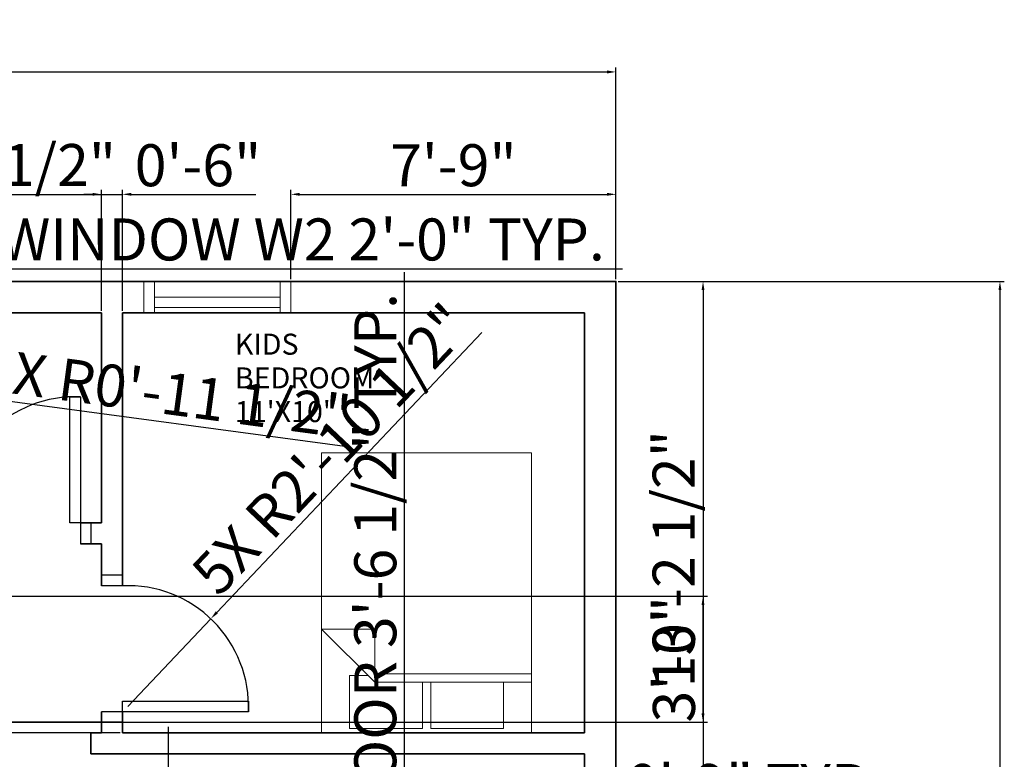
# Model space of a CAD drawing. Units: inches. Extents: x 2330 to 2931, y 514 to 1098.
# Tile 4 of 4: x 2583 to 2865, y 885 to 1096. Entities that reach past the tile are written whole.
import ezdxf

# ---------------------------------------------------------------- set-up
doc = ezdxf.new("R2010")
doc.units = ezdxf.units.IN
for name, color, linetype, lineweight in [('A-ANNO-DIMS', 2, 'Continuous', 18), ('A-AREA-IDEN', 7, 'Continuous', 18), ('A-DOOR', 3, 'Continuous', 25), ('A-FURN', 8, 'Continuous', 18), ('A-GLAZ', 4, 'Continuous', 18), ('A-WALL', 7, 'Continuous', 35)]:
    doc.layers.add(name, color=color, linetype=linetype, lineweight=lineweight)
doc.styles.get("Standard").update_dxf_attribs({"font": 'arial.ttf'})
doc.dimstyles.new('ISO-25', dxfattribs={"dimtxt": 12, "dimasz": 2.5, "dimexe": 1.25, "dimexo": 0.625, "dimtad": 1, "dimdec": 1, "dimlunit": 3, "dimtxsty": 'Standard', "dimcen": 2.5, "dimadec": 0, "dimazin": 0, "dimtfac": 1, "dimtdec": 1, "dimtmove": 0, "dimatfit": 3, "dimfxl": 1, "dimarcsym": 0})

# ---------------------------------------------------------------- blocks, each defined once
blk = doc.blocks.new('*D1')
at = {"layer": 'A-ANNO-DIMS', "color": 0, "lineweight": -2, "transparency": 16777216}
for p, q in [((2381.8, 1022.1), (2381.8, 1082.6)), ((2384.3, 1081.35), (2751.3, 1081.35)), ((2753.8, 1022.1), (2753.8, 1082.6))]:
    blk.add_line(p, q, dxfattribs=at)
at = {"layer": 'A-ANNO-DIMS', "color": 0, "transparency": 16777216}
for points in [[(2384.3, 1081.77), (2384.3, 1080.93), (2381.8, 1081.35)], [(2751.3, 1081.77), (2751.3, 1080.93), (2753.8, 1081.35)]]:
    blk.add_solid(points, dxfattribs=at)
at = {"layer": 'Defpoints', "color": 0, "transparency": 16777216}
for p in [(2753.8, 1081.35), (2381.8, 1021.47), (2753.8, 1021.47)]:
    blk.add_point(p, dxfattribs=at)
at = {"layer": 'A-ANNO-DIMS', "color": 0, "transparency": 16777216, "insert": (2567.8, 1088.11), "char_height": 12, "attachment_point": 5}
blk.add_mtext("31'", dxfattribs=at)
blk = doc.blocks.new('*D2')
at = {"layer": 'A-ANNO-DIMS', "color": 0, "lineweight": -2, "transparency": 16777216}
for p, q in [((2754.43, 1021.47), (2864.79, 1021.47)), ((2863.54, 1018.97), (2863.54, 600.97)), ((2754.43, 598.47), (2864.79, 598.47))]:
    blk.add_line(p, q, dxfattribs=at)
at = {"layer": 'A-ANNO-DIMS', "color": 0, "transparency": 16777216}
for points in [[(2863.12, 1018.97), (2863.96, 1018.97), (2863.54, 1021.47)], [(2863.12, 600.97), (2863.96, 600.97), (2863.54, 598.47)]]:
    blk.add_solid(points, dxfattribs=at)
at = {"layer": 'Defpoints', "color": 0, "transparency": 16777216}
for p in [(2753.8, 1021.47), (2753.8, 598.47), (2863.54, 598.47)]:
    blk.add_point(p, dxfattribs=at)
at = {"layer": 'A-ANNO-DIMS', "color": 0, "transparency": 16777216, "insert": (2856.78, 809.97), "char_height": 12, "attachment_point": 5, "rotation": 90}
blk.add_mtext('35\'-3"', dxfattribs=at)
blk = doc.blocks.new('Bed - Queen')
for p, q in [((0, -80.00003), (0, 0)), ((0, 0), (59.99999, 0)), ((59.99999, 0), (59.99999, -80.00003)), ((7.99999, -1.2), (28.79998, -1.2)), ((7.99999, -14.4), (7.99999, -1.2)), ((28.79998, -1.2), (28.79998, -14.4)), ((31.19999, -1.2), (51.99999, -1.2)), ((31.19999, -14.4), (31.19999, -1.2)), ((51.99999, -1.2), (51.99999, -16.4)), ((0, -14.4), (44.8, -14.4)), ((44.8, -16.8), (0, -16.8)), ((59.99999, -29.6), (44.8, -14.4)), ((44.8, -14.4), (44.8, -29.6)), ((51.99999, -16.4), (46.79936, -16.4)), ((44.8, -29.6), (59.99999, -29.6)), ((59.99999, -80.00003), (0, -80.00003))]:
    blk.add_line(p, q)
blk = doc.blocks.new('DOOR-SWING-36IN')
for p, q in [((0, 6), (0, 0)), ((3, 6), (3, 0)), ((39, 6), (39, 0)), ((42, 6), (42, 0))]:
    blk.add_line(p, q)
blk.add_lwpolyline([(39, 6), (36, 6), (36, 42), (39, 42)], close=True)
blk.add_arc((37.5, 7.5), 34.53, 87.5104, 182.4896)
blk = doc.blocks.new('WIN-36IN')
for p, q in [((0, 9), (0, 0)), ((39, 9), (3, 9)), ((3, 9), (3, 0)), ((39, 0), (39, 9)), ((42, 0), (42, 9)), ((3, 4.5), (39, 4.5)), ((3, 1.5), (39, 1.5)), ((3, 0), (39, 0))]:
    blk.add_line(p, q)
blk = doc.blocks.new('*D15')
at = {"layer": 'A-ANNO-DIMS', "color": 0, "lineweight": -2, "transparency": 16777216}
for p, q in [((2693.44, 802.89), (2693.44, 1024.11)), ((2699.18, 802.89), (2692.19, 802.89)), ((2693.44, 762.97), (2693.44, 800.39)), ((2699.18, 760.47), (2692.19, 760.47))]:
    blk.add_line(p, q, dxfattribs=at)
at = {"layer": 'A-ANNO-DIMS', "color": 0, "transparency": 16777216}
for points in [[(2693.02, 800.39), (2693.86, 800.39), (2693.44, 802.89)], [(2693.02, 762.97), (2693.86, 762.97), (2693.44, 760.47)]]:
    blk.add_solid(points, dxfattribs=at)
at = {"layer": 'Defpoints', "color": 0, "transparency": 16777216}
for p in [(2693.44, 802.89), (2699.8, 802.89), (2699.8, 760.47)]:
    blk.add_point(p, dxfattribs=at)
at = {"layer": 'A-ANNO-DIMS', "color": 0, "transparency": 16777216, "insert": (2686.6, 914.75), "char_height": 12, "attachment_point": 5, "rotation": 90}
blk.add_mtext('SWING DOOR 3\'-6 1/2" TYP.', dxfattribs=at)
blk = doc.blocks.new('*D18')
at = {"layer": 'A-ANNO-DIMS', "color": 0, "lineweight": -2, "transparency": 16777216}
for p, q in [((2744.8, 863.55), (2744.8, 870.47)), ((2753.8, 863.55), (2753.8, 870.47)), ((2747.3, 869.22), (2751.3, 869.22)), ((2753.8, 869.22), (2830.7, 869.22))]:
    blk.add_line(p, q, dxfattribs=at)
at = {"layer": 'A-ANNO-DIMS', "color": 0, "transparency": 16777216}
for points in [[(2747.3, 869.64), (2747.3, 868.8), (2744.8, 869.22)], [(2751.3, 869.64), (2751.3, 868.8), (2753.8, 869.22)]]:
    blk.add_solid(points, dxfattribs=at)
at = {"layer": 'Defpoints', "color": 0, "transparency": 16777216}
for p in [(2753.8, 869.22), (2744.8, 862.92), (2753.8, 862.92)]:
    blk.add_point(p, dxfattribs=at)
at = {"layer": 'A-ANNO-DIMS', "color": 0, "transparency": 16777216, "insert": (2793.5, 875.97), "char_height": 12, "attachment_point": 5}
blk.add_mtext('0\'-9" TYP.', dxfattribs=at)
blk = doc.blocks.new('*D19')
at = {"layer": 'A-ANNO-DIMS', "color": 0, "lineweight": -2, "transparency": 16777216}
for p, q in [((2546.27, 1022.1), (2546.27, 1026.32)), ((2548.77, 1025.07), (2567.77, 1025.07)), ((2570.27, 1022.1), (2570.27, 1026.32)), ((2570.27, 1025.07), (2755.68, 1025.07))]:
    blk.add_line(p, q, dxfattribs=at)
at = {"layer": 'A-ANNO-DIMS', "color": 0, "transparency": 16777216}
for points in [[(2548.77, 1025.49), (2548.77, 1024.66), (2546.27, 1025.07)], [(2567.77, 1025.49), (2567.77, 1024.66), (2570.27, 1025.07)]]:
    blk.add_solid(points, dxfattribs=at)
at = {"layer": 'Defpoints', "color": 0, "transparency": 16777216}
for p in [(2570.27, 1025.07), (2546.27, 1021.47), (2570.27, 1021.47)]:
    blk.add_point(p, dxfattribs=at)
at = {"layer": 'A-ANNO-DIMS', "color": 0, "transparency": 16777216, "insert": (2664.23, 1031.91), "char_height": 12, "attachment_point": 5}
blk.add_mtext('WINDOW W2 2\'-0" TYP.', dxfattribs=at)
blk = doc.blocks.new('*D39')
at = {"layer": 'A-ANNO-DIMS', "color": 0, "lineweight": -2, "transparency": 16777216}
for p, q in [((2606.8, 1013.1), (2606.8, 1047.61)), ((2612.8, 1013.1), (2612.8, 1047.61)), ((2604.3, 1046.36), (2601.8, 1046.36)), ((2606.8, 1046.36), (2612.8, 1046.36)), ((2615.3, 1046.36), (2650.95, 1046.36))]:
    blk.add_line(p, q, dxfattribs=at)
at = {"layer": 'A-ANNO-DIMS', "color": 0, "transparency": 16777216}
for points in [[(2604.3, 1046.78), (2604.3, 1045.95), (2606.8, 1046.36)], [(2615.3, 1046.78), (2615.3, 1045.95), (2612.8, 1046.36)]]:
    blk.add_solid(points, dxfattribs=at)
at = {"layer": 'Defpoints', "color": 0, "transparency": 16777216}
for p in [(2612.8, 1046.36), (2606.8, 1012.47), (2612.8, 1012.47)]:
    blk.add_point(p, dxfattribs=at)
at = {"layer": 'A-ANNO-DIMS', "color": 0, "transparency": 16777216, "insert": (2634.38, 1053.12), "char_height": 12, "attachment_point": 5}
blk.add_mtext('0\'-6"', dxfattribs=at)
blk = doc.blocks.new('*D40')
at = {"layer": 'A-ANNO-DIMS', "color": 0, "lineweight": -2, "transparency": 16777216}
for p, q in [((2528.8, 1013.1), (2528.8, 1047.61)), ((2546.27, 1013.1), (2546.27, 1047.61)), ((2531.3, 1046.36), (2543.77, 1046.36)), ((2546.27, 1046.36), (2608.76, 1046.36))]:
    blk.add_line(p, q, dxfattribs=at)
at = {"layer": 'A-ANNO-DIMS', "color": 0, "transparency": 16777216}
for points in [[(2531.3, 1046.78), (2531.3, 1045.95), (2528.8, 1046.36)], [(2543.77, 1046.78), (2543.77, 1045.95), (2546.27, 1046.36)]]:
    blk.add_solid(points, dxfattribs=at)
at = {"layer": 'Defpoints', "color": 0, "transparency": 16777216}
for p in [(2546.27, 1046.36), (2528.8, 1012.47), (2546.27, 1012.47)]:
    blk.add_point(p, dxfattribs=at)
at = {"layer": 'A-ANNO-DIMS', "color": 0, "transparency": 16777216, "insert": (2578.76, 1053.19), "char_height": 12, "attachment_point": 5}
blk.add_mtext('1\'-5 1/2"', dxfattribs=at)
blk = doc.blocks.new('*D41')
at = {"layer": 'A-ANNO-DIMS', "color": 0, "lineweight": -2, "transparency": 16777216}
for p, q in [((2660.91, 1022.1), (2660.91, 1047.61)), ((2753.8, 1022.1), (2753.8, 1047.61)), ((2663.41, 1046.36), (2751.3, 1046.36))]:
    blk.add_line(p, q, dxfattribs=at)
at = {"layer": 'A-ANNO-DIMS', "color": 0, "transparency": 16777216}
for points in [[(2663.41, 1046.78), (2663.41, 1045.95), (2660.91, 1046.36)], [(2751.3, 1046.78), (2751.3, 1045.95), (2753.8, 1046.36)]]:
    blk.add_solid(points, dxfattribs=at)
at = {"layer": 'Defpoints', "color": 0, "transparency": 16777216}
for p in [(2753.8, 1046.36), (2660.91, 1021.47), (2753.8, 1021.47)]:
    blk.add_point(p, dxfattribs=at)
at = {"layer": 'A-ANNO-DIMS', "color": 0, "transparency": 16777216, "insert": (2707.36, 1053.12), "char_height": 12, "attachment_point": 5}
blk.add_mtext('7\'-9"', dxfattribs=at)
blk = doc.blocks.new('*D46')
at = {"layer": 'A-ANNO-DIMS', "color": 0, "lineweight": -2, "transparency": 16777216}
for p, q in [((2754.43, 1021.47), (2779.95, 1021.47)), ((2778.7, 1018.97), (2778.7, 865.42)), ((2754.43, 862.92), (2779.95, 862.92))]:
    blk.add_line(p, q, dxfattribs=at)
at = {"layer": 'A-ANNO-DIMS', "color": 0, "transparency": 16777216}
for points in [[(2778.28, 1018.97), (2779.11, 1018.97), (2778.7, 1021.47)], [(2778.28, 865.42), (2779.11, 865.42), (2778.7, 862.92)]]:
    blk.add_solid(points, dxfattribs=at)
at = {"layer": 'Defpoints', "color": 0, "transparency": 16777216}
for p in [(2753.8, 1021.47), (2753.8, 862.92), (2778.7, 862.92)]:
    blk.add_point(p, dxfattribs=at)
at = {"layer": 'A-ANNO-DIMS', "color": 0, "transparency": 16777216, "insert": (2771.86, 942.2), "char_height": 12, "attachment_point": 5, "rotation": 90}
blk.add_mtext('13\'-2 1/2"', dxfattribs=at)
blk = doc.blocks.new('*D53')
at = {"layer": 'A-ANNO-DIMS', "color": 0, "lineweight": -2, "transparency": 16777216}
for p, q in [((2523.43, 931.47), (2779.95, 931.47)), ((2778.7, 897.97), (2778.7, 928.97)), ((2523.43, 895.47), (2779.95, 895.47))]:
    blk.add_line(p, q, dxfattribs=at)
at = {"layer": 'A-ANNO-DIMS', "color": 0, "transparency": 16777216}
for points in [[(2778.28, 928.97), (2779.11, 928.97), (2778.7, 931.47)], [(2778.28, 897.97), (2779.11, 897.97), (2778.7, 895.47)]]:
    blk.add_solid(points, dxfattribs=at)
at = {"layer": 'Defpoints', "color": 0, "transparency": 16777216}
for p in [(2522.8, 931.47), (2778.7, 931.47), (2522.8, 895.47)]:
    blk.add_point(p, dxfattribs=at)
at = {"layer": 'A-ANNO-DIMS', "color": 0, "transparency": 16777216, "insert": (2771.94, 913.47), "char_height": 12, "attachment_point": 5, "rotation": 90}
blk.add_mtext('3\'-0"', dxfattribs=at)
blk = doc.blocks.new('*D56')
at = {"layer": 'A-ANNO-DIMS', "color": 0, "lineweight": -2, "transparency": 16777216}
for p, q in [((2528.8, 945.85), (2528.8, 572.33)), ((2561.8, 945.85), (2561.8, 572.33)), ((2531.3, 573.58), (2559.3, 573.58)), ((2561.8, 573.58), (2597.66, 573.58))]:
    blk.add_line(p, q, dxfattribs=at)
at = {"layer": 'A-ANNO-DIMS', "color": 0, "transparency": 16777216}
for points in [[(2531.3, 574), (2531.3, 573.16), (2528.8, 573.58)], [(2559.3, 574), (2559.3, 573.16), (2561.8, 573.58)]]:
    blk.add_solid(points, dxfattribs=at)
at = {"layer": 'Defpoints', "color": 0, "transparency": 16777216}
for p in [(2528.8, 946.47), (2561.8, 946.47), (2561.8, 573.58)]:
    blk.add_point(p, dxfattribs=at)
at = {"layer": 'A-ANNO-DIMS', "color": 0, "transparency": 16777216, "insert": (2580.98, 580.33), "char_height": 12, "attachment_point": 5}
blk.add_mtext('2\'-9"', dxfattribs=at)
blk = doc.blocks.new('*D57')
at = {"layer": 'A-ANNO-DIMS', "color": 0, "lineweight": -2, "transparency": 16777216}
for p, q in [((2356.91, 897.97), (2356.91, 933.62)), ((2612.18, 895.47), (2355.66, 895.47)), ((2356.91, 892.47), (2356.91, 895.47)), ((2612.18, 892.47), (2355.66, 892.47)), ((2356.91, 889.97), (2356.91, 887.47))]:
    blk.add_line(p, q, dxfattribs=at)
at = {"layer": 'A-ANNO-DIMS', "color": 0, "transparency": 16777216}
for points in [[(2356.49, 897.97), (2357.33, 897.97), (2356.91, 895.47)], [(2356.49, 889.97), (2357.33, 889.97), (2356.91, 892.47)]]:
    blk.add_solid(points, dxfattribs=at)
at = {"layer": 'Defpoints', "color": 0, "transparency": 16777216}
for p in [(2356.91, 895.47), (2612.8, 895.47), (2612.8, 892.47)]:
    blk.add_point(p, dxfattribs=at)
at = {"layer": 'A-ANNO-DIMS', "color": 0, "transparency": 16777216, "insert": (2350.15, 917.05), "char_height": 12, "attachment_point": 5, "rotation": 90}
blk.add_mtext('0\'-3"', dxfattribs=at)
blk = doc.blocks.new('*D58')
at = {"layer": 'A-ANNO-DIMS', "color": 0, "lineweight": -2, "transparency": 16777216}
for p, q in [((2715.53, 1006.89), (2639.76, 926.86)), ((2614.3, 899.97), (2638.05, 925.05))]:
    blk.add_line(p, q, dxfattribs=at)
at = {"layer": 'A-ANNO-DIMS', "color": 0, "transparency": 16777216}
blk.add_solid([(2639.46, 927.15), (2640.07, 926.58), (2638.05, 925.05)], dxfattribs=at)
at = {"layer": 'Defpoints', "color": 0, "transparency": 16777216}
for p in [(2638.05, 925.05), (2614.3, 899.97)]:
    blk.add_point(p, dxfattribs=at)
at = {"layer": 'A-ANNO-DIMS', "color": 0, "transparency": 16777216, "insert": (2673.55, 972.48), "char_height": 12, "attachment_point": 5, "rotation": 46.5643}
blk.add_mtext('5X R2\'-10 1/2"', dxfattribs=at)
blk = doc.blocks.new('*D59')
at = {"layer": 'A-ANNO-DIMS', "color": 0, "lineweight": -2, "transparency": 16777216}
for p, q in [((2625.86, 894.18), (2625.87, 772.98)), ((2625.87, 673.28), (2625.87, 770.48))]:
    blk.add_line(p, q, dxfattribs=at)
at = {"layer": 'A-ANNO-DIMS', "color": 0, "transparency": 16777216}
blk.add_solid([(2626.28, 770.48), (2625.45, 770.48), (2625.87, 772.98)], dxfattribs=at)
at = {"layer": 'Defpoints', "color": 0, "transparency": 16777216}
for p in [(2625.86, 894.18), (2625.87, 772.98)]:
    blk.add_point(p, dxfattribs=at)
at = {"layer": 'A-ANNO-DIMS', "color": 0, "transparency": 16777216, "insert": (2632.62, 700.26), "char_height": 12, "attachment_point": 5, "rotation": 270.0001}
blk.add_mtext('R10\'-1"', dxfattribs=at)
blk = doc.blocks.new('*D64')
at = {"layer": 'A-ANNO-DIMS', "color": 0, "lineweight": -2, "transparency": 16777216}
for p, q in [((2554.35, 990.65), (2565.58, 989.14)), ((2677.75, 974.06), (2568.05, 988.81))]:
    blk.add_line(p, q, dxfattribs=at)
at = {"layer": 'A-ANNO-DIMS', "color": 0, "transparency": 16777216}
blk.add_solid([(2568.11, 989.22), (2568, 988.4), (2565.58, 989.14)], dxfattribs=at)
at = {"layer": 'Defpoints', "color": 0, "transparency": 16777216}
for p in [(2554.35, 990.65), (2565.58, 989.14)]:
    blk.add_point(p, dxfattribs=at)
at = {"layer": 'A-ANNO-DIMS', "color": 0, "transparency": 16777216, "insert": (2625.05, 988.04), "char_height": 12, "attachment_point": 5, "rotation": 352.3416}
blk.add_mtext('4X R0\'-11 1/2"', dxfattribs=at)

msp = doc.modelspace()

# ---------------------------------------------------------------- linework, layer by layer
at = {"layer": 'A-WALL'}
for p, q in [((2606.8, 1012.47), (2528.8, 1012.47)), ((2606.8, 952.47), (2606.8, 1012.47)), ((2744.8, 1012.47), (2612.8, 1012.47)), ((2612.8, 934.47), (2612.8, 1012.47)), ((2744.8, 892.47), (2744.8, 1012.47)), ((2606.8, 952.47), (2600.8, 952.47)), ((2606.8, 946.47), (2600.8, 946.47)), ((2606.8, 934.47), (2606.8, 946.47)), ((2606.8, 892.47), (2606.8, 898.47)), ((2612.8, 892.47), (2612.8, 898.47)), ((2606.8, 892.47), (2603.8, 892.47)), ((2603.8, 892.47), (2603.8, 886.47)), ((2744.8, 892.47), (2612.8, 892.47)), ((2606.8, 886.47), (2603.8, 886.47)), ((2744.8, 886.47), (2606.8, 886.47)), ((2744.8, 766.47), (2744.8, 886.47))]:
    msp.add_line(p, q, dxfattribs=at)
msp.add_lwpolyline([(2738.8, 598.47), (2753.8, 598.47), (2753.8, 1021.47), (2381.8, 1021.47), (2381.8, 598.47), (2624.83, 598.47)], dxfattribs=at)

# ---------------------------------------------------------------- block references
at = {"layer": 'A-DOOR'}
msp.add_blockref('DOOR-SWING-36IN', (2561.8, 946.47), dxfattribs=at)
at = {"layer": 'A-DOOR', "rotation": 270.0000000000019}
msp.add_blockref('DOOR-SWING-36IN', (2606.8, 937.47), dxfattribs=at)
at = {"layer": 'A-FURN', "rotation": 180}
msp.add_blockref('Bed - Queen', (2729.7, 892.47), dxfattribs=at)
at = {"layer": 'A-GLAZ'}
msp.add_blockref('WIN-36IN', (2618.91, 1012.47), dxfattribs=at)

# ---------------------------------------------------------------- texts
at = {"layer": 'A-AREA-IDEN'}
for s, p in [('KIDS', (2644.93, 1000.53)), ('BEDROOM', (2644.93, 990.89)), ("11'X10'", (2644.93, 981.25))]:
    msp.add_text(s, height=6, dxfattribs=at).set_placement(p)

# ---------------------------------------------------------------- dimensions: what is measured, and where the dimension line sits
at = {"layer": 'A-ANNO-DIMS'}
for base, p1, p2, override, picture, middle in [((2753.8, 1081.35), (2381.8, 1021.47), (2753.8, 1021.47), {"dimclrd": 0, "dimclre": 0, "dimclrt": 0}, '*D1', (2567.8, 1088.11)), ((2546.27, 1046.36), (2528.8, 1012.47), (2546.27, 1012.47), {"dimdec": 1, "dimlfac": 1, "dimrnd": 0, "dimzin": 1, "dimdsep": 46, "dimlunit": 4, "dimfrac": 2}, '*D40', (2578.76, 1053.19)), ((2612.8, 1046.36), (2606.8, 1012.47), (2612.8, 1012.47), {"dimdec": 1, "dimlfac": 1, "dimrnd": 0, "dimzin": 1, "dimdsep": 46, "dimlunit": 4, "dimfrac": 2}, '*D39', (2634.38, 1053.12)), ((2753.8, 1046.36), (2660.91, 1021.47), (2753.8, 1021.47), {"dimdec": 1, "dimlfac": 1, "dimrnd": 0, "dimzin": 1, "dimdsep": 46, "dimlunit": 4, "dimfrac": 2}, '*D41', (2707.36, 1053.12)), ((2561.8, 573.58), (2528.8, 946.47), (2561.8, 946.47), {"dimdec": 1, "dimlfac": 1, "dimrnd": 0, "dimzin": 1, "dimdsep": 46, "dimlunit": 4, "dimfrac": 2}, '*D56', (2580.98, 580.33))]:
    dim = msp.add_linear_dim(base=base, p1=p1, p2=p2, dimstyle='ISO-25', override=override, dxfattribs=at)
    dim.commit()
    dim.dimension.update_dxf_attribs({"geometry": picture, "text_midpoint": middle})
dim = msp.add_linear_dim(base=(2570.27, 1025.07), p1=(2546.27, 1021.47), p2=(2570.27, 1021.47), text='WINDOW W2 <> TYP.', dimstyle='ISO-25', override={"dimdec": 1, "dimlfac": 1, "dimrnd": 0, "dimzin": 1, "dimdsep": 46, "dimlunit": 4, "dimfrac": 2}, dxfattribs=at)
dim.commit()
dim.dimension.update_dxf_attribs({"geometry": '*D19', "text_midpoint": (2664.23, 1031.91)})
for base, p1, p2, angle, text, picture, middle in [((2693.44, 802.89), (2699.8, 760.47), (2699.8, 802.89), 90, 'SWING DOOR <> TYP.', '*D15', (2686.6, 914.75)), ((2753.8, 869.22), (2744.8, 862.92), (2753.8, 862.92), 0, '<> TYP.', '*D18', (2793.5, 875.97))]:
    dim = msp.add_linear_dim(base=base, p1=p1, p2=p2, angle=angle, text=text, dimstyle='ISO-25', override={"dimdec": 1, "dimlfac": 1, "dimrnd": 0, "dimzin": 1, "dimdsep": 46, "dimlunit": 4, "dimfrac": 2}, dxfattribs=at)
    dim.commit()
    dim.dimension.update_dxf_attribs({"geometry": picture, "text_midpoint": middle})
for base, p1, p2, override, picture, middle in [((2863.54, 598.47), (2753.8, 1021.47), (2753.8, 598.47), {"dimclrd": 0, "dimclre": 0, "dimclrt": 0}, '*D2', (2856.78, 809.97)), ((2778.6953, 862.9209), (2753.8028, 1021.4722), (2753.8028, 862.9209), {"dimdec": 1, "dimlfac": 1, "dimrnd": 0, "dimzin": 1, "dimdsep": 46, "dimlunit": 4, "dimfrac": 2}, '*D46', (2771.8615, 942.1965)), ((2356.91, 895.47), (2612.8, 892.47), (2612.8, 895.47), {"dimdec": 1, "dimlfac": 1, "dimrnd": 0, "dimzin": 1, "dimdsep": 46, "dimlunit": 4, "dimfrac": 2}, '*D57', (2350.15, 917.05)), ((2778.7, 931.47), (2522.8, 895.47), (2522.8, 931.47), {"dimdec": 1, "dimlfac": 1, "dimrnd": 0, "dimzin": 1, "dimdsep": 46, "dimlunit": 4, "dimfrac": 2}, '*D53', (2771.94, 913.47))]:
    dim = msp.add_linear_dim(base=base, p1=p1, p2=p2, angle=90, dimstyle='ISO-25', override=override, dxfattribs=at)
    dim.commit()
    dim.dimension.update_dxf_attribs({"geometry": picture, "text_midpoint": middle})
for center, mpoint, text, picture, middle in [((2554.35, 990.65), (2565.58, 989.14), '4X <>', '*D64', (2625.05, 988.04)), ((2614.3, 899.97), (2638.05, 925.05), '5X <>', '*D58', (2673.55, 972.48))]:
    dim = msp.add_radius_dim(center=center, mpoint=mpoint, text=text, dimstyle='ISO-25', override={"dimdec": 1, "dimlfac": 1, "dimrnd": 0, "dimzin": 1, "dimdsep": 46, "dimlunit": 4, "dimfrac": 2}, dxfattribs=at)
    dim.commit()
    dim.dimension.update_dxf_attribs({"geometry": picture, "text_midpoint": middle})
dim = msp.add_radius_dim(center=(2625.86, 894.18), mpoint=(2625.87, 772.98), dimstyle='ISO-25', override={"dimdec": 1, "dimlfac": 1, "dimrnd": 0, "dimzin": 1, "dimdsep": 46, "dimlunit": 4, "dimfrac": 2}, dxfattribs=at)
dim.commit()
dim.dimension.update_dxf_attribs({"geometry": '*D59', "text_midpoint": (2625.87, 700.26), "dimtype": 164})

doc.saveas('drawing.dxf')
